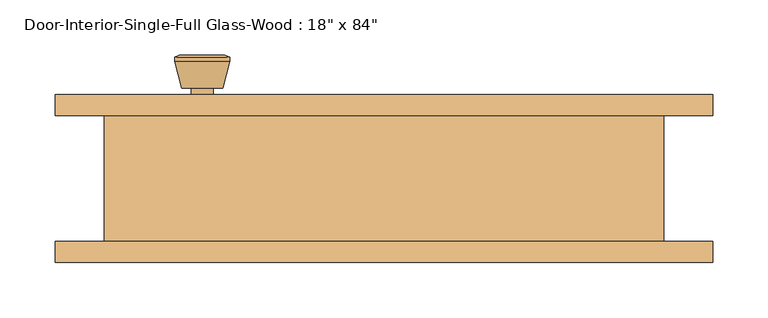
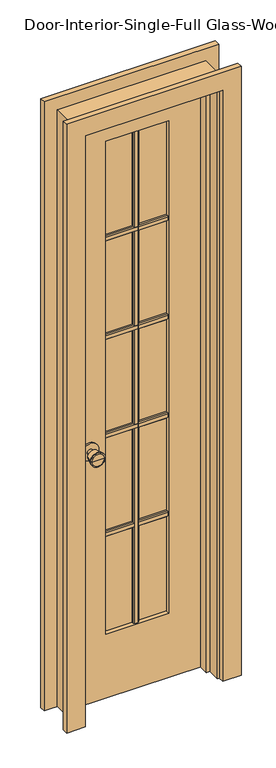
"""IFC4 building model written with IfcOpenShell, lengths in millimetres: door geometry."""

from ifc_helpers import new_model, si_unit, point, frame, frame_2d, origin, place, context, project, spatial, polyline, circle_curve, trimmed, segment, composite_curve, outline, extrude, faceted_brep, source, transform, mapped, element, save
from ifc_brep_helpers import plane_surface, cylinder_surface, revolved_surface, advanced_brep


def door_ccf0cbd1(model_context):
    return source(origin(), model_context, "Body", "SolidModel", [
        extrude(outline(polyline([(40.005, 1667.51), (46.355, 1667.51), (49.53, 1664.335), (49.53, 1651.635), (46.355, 1648.46), (40.005, 1648.46), (40.005, 1667.51)])), frame((-107.95, 0.0, 0.0), z_axis=(1.0, 0.0, 0.0), x_axis=(0.0, 1.0, 0.0)), (0.0, 0.0, 1.0), 215.9),
        extrude(outline(polyline([(40.005, 1310.9575), (46.355, 1310.9575), (49.53, 1307.7825), (49.53, 1295.0825), (46.355, 1291.9075), (40.005, 1291.9075), (40.005, 1310.9575)])), frame((-107.95, 0.0, 0.0), z_axis=(1.0, 0.0, 0.0), x_axis=(0.0, 1.0, 0.0)), (0.0, 0.0, 1.0), 215.9),
        extrude(outline(polyline([(40.005, 954.405), (46.355, 954.405), (49.53, 951.23), (49.53, 938.53), (46.355, 935.355), (40.005, 935.355), (40.005, 954.405)])), frame((-107.95, 0.0, 0.0), z_axis=(1.0, 0.0, 0.0), x_axis=(0.0, 1.0, 0.0)), (0.0, 0.0, 1.0), 215.9),
        extrude(outline(polyline([(-9.525, 40.005), (-9.525, 46.355), (-6.35, 49.53), (6.35, 49.53), (9.525, 46.355), (9.525, 40.005), (-9.525, 40.005)])), frame((0.0, 0.0, 231.775), z_axis=(0.0, 0.0, 1.0), x_axis=(1.0, 0.0, 0.0)), (0.0, 0.0, 1.0), 1782.7625),
        extrude(outline(polyline([(40.005, 597.8525), (46.355, 597.8525), (49.53, 594.6775), (49.53, 581.9775), (46.355, 578.8025), (40.005, 578.8025), (40.005, 597.8525)])), frame((-107.95, 0.0, 0.0), z_axis=(1.0, 0.0, 0.0), x_axis=(0.0, 1.0, 0.0)), (0.0, 0.0, 1.0), 215.9),
        extrude(outline(polyline([(33.02, 1667.51), (33.02, 1648.46), (26.67, 1648.46), (23.495, 1651.635), (23.495, 1664.335), (26.67, 1667.51), (33.02, 1667.51)])), frame((-107.95, 0.0, 0.0), z_axis=(1.0, 0.0, 0.0), x_axis=(0.0, 1.0, 0.0)), (0.0, 0.0, 1.0), 215.9),
        extrude(outline(polyline([(33.02, 1310.9575), (33.02, 1291.9075), (26.67, 1291.9075), (23.495, 1295.0825), (23.495, 1307.7825), (26.67, 1310.9575), (33.02, 1310.9575)])), frame((-107.95, 0.0, 0.0), z_axis=(1.0, 0.0, 0.0), x_axis=(0.0, 1.0, 0.0)), (0.0, 0.0, 1.0), 215.9),
        extrude(outline(polyline([(33.02, 954.405), (33.02, 935.355), (26.67, 935.355), (23.495, 938.53), (23.495, 951.23), (26.67, 954.405), (33.02, 954.405)])), frame((-107.95, 0.0, 0.0), z_axis=(1.0, 0.0, 0.0), x_axis=(0.0, 1.0, 0.0)), (0.0, 0.0, 1.0), 215.9),
        extrude(outline(polyline([(-9.525, 33.02), (9.525, 33.02), (9.525, 26.67), (6.35, 23.495), (-6.35, 23.495), (-9.525, 26.67), (-9.525, 33.02)])), frame((0.0, 0.0, 231.775), z_axis=(0.0, 0.0, 1.0), x_axis=(1.0, 0.0, 0.0)), (0.0, 0.0, 1.0), 1782.7625),
        extrude(outline(polyline([(33.02, 597.8525), (33.02, 578.8025), (26.67, 578.8025), (23.495, 581.9775), (23.495, 594.6775), (26.67, 597.8525), (33.02, 597.8525)])), frame((-107.95, 0.0, 0.0), z_axis=(1.0, 0.0, 0.0), x_axis=(0.0, 1.0, 0.0)), (0.0, 0.0, 1.0), 215.9),
        advanced_brep(
        [(-165.1, 13.05, 914.4), (-155.1, 13.05, 914.4), (-175.1, 13.05, 914.4), (-144.6241324, -35.95, 914.4), (-165.1, -35.95, 914.4), (-185.5758676, -35.95, 914.4), (-140.1, -34.1221319, 914.4), (-190.1, -34.1221319, 914.4), (-140.1, -30.6584537, 914.4), (-190.1, -30.6584537, 914.4), (-146.463764, -5.95, 914.4), (-183.736236, -5.95, 914.4), (-155.1, -5.95, 914.4), (-175.1, -5.95, 914.4)],
        [
            (0, 1),
            (1, 2, circle_curve(frame((-165.1, 13.05, 914.4), z_axis=(0.0, 1.0, 0.0), x_axis=(-1.0, 0.0, 0.0)), 10.0)),
            (2, 0),
            (2, 1, circle_curve(frame((-165.1, 13.05, 914.4), z_axis=(0.0, 1.0, 0.0), x_axis=(-1.0, 0.0, 0.0)), 10.0)),
            (3, 4),
            (4, 5),
            (5, 3, circle_curve(frame((-165.1, -35.95, 914.4), z_axis=(0.0, -1.0, 0.0), x_axis=(-1.0, 0.0, 0.0)), 20.4758676)),
            (3, 5, circle_curve(frame((-165.1, -35.95, 914.4), z_axis=(0.0, -1.0, 0.0), x_axis=(-1.0, 0.0, 0.0)), 20.4758676)),
            (6, 3),
            (5, 7),
            (7, 6, circle_curve(frame((-165.1, -34.1221319, 914.4), z_axis=(0.0, -1.0, 0.0), x_axis=(-1.0, 0.0, 0.0)), 25.0)),
            (6, 7, circle_curve(frame((-165.1, -34.1221319, 914.4), z_axis=(0.0, -1.0, 0.0), x_axis=(-1.0, 0.0, 0.0)), 25.0)),
            (8, 6),
            (7, 9),
            (9, 8, circle_curve(frame((-165.1, -30.6584537, 914.4), z_axis=(0.0, -1.0, 0.0), x_axis=(-1.0, 0.0, 0.0)), 25.0)),
            (8, 9, circle_curve(frame((-165.1, -30.6584537, 914.4), z_axis=(0.0, -1.0, 0.0), x_axis=(-1.0, 0.0, 0.0)), 25.0)),
            (10, 8),
            (9, 11),
            (11, 10, circle_curve(frame((-165.1, -5.95, 914.4), z_axis=(0.0, -1.0, 0.0), x_axis=(-1.0, 0.0, 0.0)), 18.636236)),
            (10, 11, circle_curve(frame((-165.1, -5.95, 914.4), z_axis=(0.0, -1.0, 0.0), x_axis=(-1.0, 0.0, 0.0)), 18.636236)),
            (12, 10),
            (11, 13),
            (13, 12, circle_curve(frame((-165.1, -5.95, 914.4), z_axis=(0.0, -1.0, 0.0), x_axis=(-1.0, 0.0, 0.0)), 10.0)),
            (12, 13, circle_curve(frame((-165.1, -5.95, 914.4), z_axis=(0.0, -1.0, 0.0), x_axis=(-1.0, 0.0, 0.0)), 10.0)),
            (1, 12),
            (13, 2),
        ],
        [
            plane_surface(frame((-165.1, 13.05, 914.4), z_axis=(0.0, 1.0, 0.0), x_axis=(-1.0, 0.0, 0.0))),
            plane_surface(frame((-165.1, -35.95, 914.4), z_axis=(0.0, -1.0, 0.0), x_axis=(-1.0, 0.0, 0.0))),
            revolved_surface(polyline([(-185.5758676, -35.95, 914.4), (-190.1, -34.1221319, 914.4)]), (-165.1, 13.05, 914.4), (0.0, 1.0, 0.0)),
            cylinder_surface(frame((-165.1, 13.05, 914.4), z_axis=(0.0, 1.0, 0.0), x_axis=(-1.0, 0.0, 0.0)), 25.0),
            revolved_surface(polyline([(-190.1, -30.6584537, 914.4), (-183.736236, -5.95, 914.4)]), (-165.1, 13.05, 914.4), (0.0, 1.0, 0.0)),
            plane_surface(frame((-165.1, -5.95, 914.4), z_axis=(0.0, 1.0, 0.0), x_axis=(-1.0, 0.0, 0.0))),
            cylinder_surface(frame((-165.1, 13.05, 914.4), z_axis=(0.0, 1.0, 0.0), x_axis=(-1.0, 0.0, 0.0)), 10.0),
        ],
        [
            (0, [[1, 2, 3]]),
            (0, [[-3, 4, -1]]),
            (1, [[5, 6, 7]]),
            (1, [[-6, -5, 8]]),
            (2, [[9, -7, 10, 11]]),
            (2, [[-10, -8, -9, 12]]),
            (3, [[13, -11, 14, 15]]),
            (3, [[-14, -12, -13, 16]]),
            (4, [[17, -15, 18, 19]]),
            (4, [[-18, -16, -17, 20]]),
            (5, [[21, -19, 22, 23]]),
            (5, [[-22, -20, -21, 24]]),
            (6, [[25, -23, 26, -2]]),
            (6, [[-26, -24, -25, -4]]),
        ],
    ),
        extrude(outline(composite_curve([segment(trimmed(circle_curve(frame_2d((914.4, -165.1)), 30.0), [point((914.4, -195.1))], [point((914.4, -135.1))], False, "CARTESIAN"), True, "CONTINUOUS"), segment(trimmed(circle_curve(frame_2d((914.4, -165.1)), 30.0), [point((914.4, -135.1))], [point((914.4, -195.1))], False, "CARTESIAN"), True, "CONTINUOUS")], self_intersect=False)), frame((0.0, 13.05, 0.0), z_axis=(0.0, 1.0, 0.0), x_axis=(0.0, 0.0, 1.0)), (0.0, 0.0, 1.0), 6.0),
        advanced_brep(
        [(-165.1, 59.975, 914.4), (-175.1, 59.975, 914.4), (-155.1, 59.975, 914.4), (-144.6241324, 108.975, 914.4), (-185.5758676, 108.975, 914.4), (-165.1, 108.975, 914.4), (-140.1, 107.1471319, 914.4), (-190.1, 107.1471319, 914.4), (-140.1, 103.6834537, 914.4), (-190.1, 103.6834537, 914.4), (-146.463764, 78.975, 914.4), (-183.736236, 78.975, 914.4), (-155.1, 78.975, 914.4), (-175.1, 78.975, 914.4)],
        [
            (0, 1),
            (1, 2, circle_curve(frame((-165.1, 59.975, 914.4), z_axis=(0.0, -1.0, 0.0), x_axis=(-1.0, 0.0, 0.0)), 10.0)),
            (2, 0),
            (2, 1, circle_curve(frame((-165.1, 59.975, 914.4), z_axis=(0.0, -1.0, 0.0), x_axis=(-1.0, 0.0, 0.0)), 10.0)),
            (3, 4, circle_curve(frame((-165.1, 108.975, 914.4), z_axis=(0.0, 1.0, 0.0), x_axis=(-1.0, 0.0, 0.0)), 20.4758676)),
            (4, 5),
            (5, 3),
            (4, 3, circle_curve(frame((-165.1, 108.975, 914.4), z_axis=(0.0, 1.0, 0.0), x_axis=(-1.0, 0.0, 0.0)), 20.4758676)),
            (6, 7, circle_curve(frame((-165.1, 107.1471319, 914.4), z_axis=(0.0, 1.0, 0.0), x_axis=(-1.0, 0.0, 0.0)), 25.0)),
            (7, 4),
            (3, 6),
            (7, 6, circle_curve(frame((-165.1, 107.1471319, 914.4), z_axis=(0.0, 1.0, 0.0), x_axis=(-1.0, 0.0, 0.0)), 25.0)),
            (8, 9, circle_curve(frame((-165.1, 103.6834537, 914.4), z_axis=(0.0, 1.0, 0.0), x_axis=(-1.0, 0.0, 0.0)), 25.0)),
            (9, 7),
            (6, 8),
            (9, 8, circle_curve(frame((-165.1, 103.6834537, 914.4), z_axis=(0.0, 1.0, 0.0), x_axis=(-1.0, 0.0, 0.0)), 25.0)),
            (10, 11, circle_curve(frame((-165.1, 78.975, 914.4), z_axis=(0.0, 1.0, 0.0), x_axis=(-1.0, 0.0, 0.0)), 18.636236)),
            (11, 9),
            (8, 10),
            (11, 10, circle_curve(frame((-165.1, 78.975, 914.4), z_axis=(0.0, 1.0, 0.0), x_axis=(-1.0, 0.0, 0.0)), 18.636236)),
            (12, 13, circle_curve(frame((-165.1, 78.975, 914.4), z_axis=(0.0, 1.0, 0.0), x_axis=(-1.0, 0.0, 0.0)), 10.0)),
            (13, 11),
            (10, 12),
            (13, 12, circle_curve(frame((-165.1, 78.975, 914.4), z_axis=(0.0, 1.0, 0.0), x_axis=(-1.0, 0.0, 0.0)), 10.0)),
            (1, 13),
            (12, 2),
        ],
        [
            plane_surface(frame((-165.1, 59.975, 914.4), z_axis=(0.0, -1.0, 0.0), x_axis=(-1.0, 0.0, 0.0))),
            plane_surface(frame((-165.1, 108.975, 914.4), z_axis=(0.0, 1.0, 0.0), x_axis=(-1.0, 0.0, 0.0))),
            revolved_surface(polyline([(-185.5758676, 108.975, 914.4), (-190.1, 107.1471319, 914.4)]), (-165.1, 59.975, 914.4), (0.0, -1.0, 0.0)),
            cylinder_surface(frame((-165.1, 59.975, 914.4), z_axis=(0.0, -1.0, 0.0), x_axis=(-1.0, 0.0, 0.0)), 25.0),
            revolved_surface(polyline([(-190.1, 103.6834537, 914.4), (-183.736236, 78.975, 914.4)]), (-165.1, 59.975, 914.4), (0.0, -1.0, 0.0)),
            plane_surface(frame((-165.1, 78.975, 914.4), z_axis=(0.0, -1.0, 0.0), x_axis=(-1.0, 0.0, 0.0))),
            cylinder_surface(frame((-165.1, 59.975, 914.4), z_axis=(0.0, -1.0, 0.0), x_axis=(-1.0, 0.0, 0.0)), 10.0),
        ],
        [
            (0, [[1, 2, 3]]),
            (0, [[-3, 4, -1]]),
            (1, [[5, 6, 7]]),
            (1, [[8, -7, -6]]),
            (2, [[9, 10, -5, 11]]),
            (2, [[12, -11, -8, -10]]),
            (3, [[13, 14, -9, 15]]),
            (3, [[16, -15, -12, -14]]),
            (4, [[17, 18, -13, 19]]),
            (4, [[20, -19, -16, -18]]),
            (5, [[21, 22, -17, 23]]),
            (5, [[24, -23, -20, -22]]),
            (6, [[-2, 25, -21, 26]]),
            (6, [[-4, -26, -24, -25]]),
        ],
    ),
        extrude(outline(composite_curve([segment(trimmed(circle_curve(frame_2d((914.4, -165.1)), 30.0), [point((914.4, -195.1))], [point((914.4, -135.1))], False, "CARTESIAN"), True, "CONTINUOUS"), segment(trimmed(circle_curve(frame_2d((914.4, -165.1)), 30.0), [point((914.4, -135.1))], [point((914.4, -195.1))], False, "CARTESIAN"), True, "CONTINUOUS")], self_intersect=False)), frame((0.0, 53.975, 0.0), z_axis=(0.0, 1.0, 0.0), x_axis=(0.0, 0.0, 1.0)), (0.0, 0.0, 1.0), 6.0),
        faceted_brep([(254.0, 53.975, 0.0), (254.0, -60.325, 0.0), (228.6, -60.325, 0.0), (228.6, -15.875, 0.0), (215.9, -15.875, 0.0), (215.9, 19.05, 0.0), (228.6, 19.05, 0.0), (228.6, 53.975, 0.0), (254.0, 53.975, 2159.0), (254.0, -60.325, 2159.0), (-254.0, -60.325, 2159.0), (-254.0, -60.325, 0.0), (-228.6, -60.325, 0.0), (-228.6, -60.325, 2133.6), (228.6, -60.325, 2133.6), (228.6, -15.875, 2133.6), (-228.6, -15.875, 2133.6), (-228.6, -15.875, 0.0), (-215.9, -15.875, 0.0), (-215.9, -15.875, 2120.9), (215.9, -15.875, 2120.9), (215.9, 19.05, 2120.9), (-215.9, 19.05, 2120.9), (-215.9, 19.05, 0.0), (-228.6, 19.05, 0.0), (-228.6, 19.05, 2133.6), (228.6, 19.05, 2133.6), (228.6, 53.975, 2133.6), (-228.6, 53.975, 2133.6), (-228.6, 53.975, 0.0), (-254.0, 53.975, 0.0), (-254.0, 53.975, 2159.0)], [[[0, 1, 2, 3, 4, 5, 6, 7]], [[1, 0, 8, 9]], [[2, 1, 9, 10, 11, 12, 13, 14]], [[3, 2, 14, 15]], [[4, 3, 15, 16, 17, 18, 19, 20]], [[5, 4, 20, 21]], [[6, 5, 21, 22, 23, 24, 25, 26]], [[7, 6, 26, 27]], [[0, 7, 27, 28, 29, 30, 31, 8]], [[9, 8, 31, 10]], [[15, 14, 13, 16]], [[21, 20, 19, 22]], [[27, 26, 25, 28]], [[30, 29, 24, 23, 18, 17, 12, 11]], [[10, 31, 30, 11]], [[16, 13, 12, 17]], [[22, 19, 18, 23]], [[28, 25, 24, 29]]]),
        extrude(outline(polyline([(2133.6, -228.6), (0.0, -228.6), (0.0, 228.6), (2133.6, 228.6), (2133.6, -228.6)]), holes=[polyline([(2014.5375, -107.95), (2014.5375, 107.95), (231.775, 107.95), (231.775, -107.95), (2014.5375, -107.95)])]), frame((0.0, 19.05, 0.0), z_axis=(0.0, 1.0, 0.0), x_axis=(0.0, 0.0, 1.0)), (0.0, 0.0, 1.0), 34.925),
        extrude(outline(polyline([(107.95, 33.02), (-107.95, 33.02), (-107.95, 40.005), (107.95, 40.005), (107.95, 33.02)])), frame((0.0, 0.0, 231.775), z_axis=(0.0, 0.0, 1.0), x_axis=(1.0, 0.0, 0.0)), (0.0, 0.0, 1.0), 1782.7625),
        extrude(outline(polyline([(0.0, 234.95), (0.0, 298.45), (2203.45, 298.45), (2203.45, -298.45), (0.0, -298.45), (0.0, -234.95), (2139.95, -234.95), (2139.95, 234.95), (0.0, 234.95)])), frame((0.0, 53.975, 0.0), z_axis=(0.0, 1.0, 0.0), x_axis=(0.0, 0.0, 1.0)), (0.0, 0.0, 1.0), 19.05),
        extrude(outline(polyline([(0.0, 234.95), (0.0, 298.45), (2203.45, 298.45), (2203.45, -298.45), (0.0, -298.45), (0.0, -234.95), (2139.95, -234.95), (2139.95, 234.95), (0.0, 234.95)])), frame((0.0, -79.375, 0.0), z_axis=(0.0, 1.0, 0.0), x_axis=(0.0, 0.0, 1.0)), (0.0, 0.0, 1.0), 19.05),
    ])


if __name__ == "__main__":
    model = new_model("IFC4")
    model_context = context("Model", 3, world=origin())
    ifc_project = project(units=[si_unit("LENGTHUNIT", "METRE", prefix="MILLI")], contexts=[model_context])
    site = spatial("IfcSite", under=ifc_project)
    building = spatial("IfcBuilding", under=site)
    placement = place(None, origin())
    door_shape = door_ccf0cbd1(model_context)
    element("IfcDoor", 1, ObjectType="Door-Interior-Single-Full Glass-Wood : 18\" x 84\"", at=placement, inside=building, context=model_context, shape_type="MappedRepresentation", body=[
        mapped(door_shape, transform((0.0, 0.0, 0.0), x_axis=(1.0, 0.0, 0.0), y_axis=(0.0, 1.0, 0.0), z_axis=(0.0, 0.0, 1.0))),
    ])
    save(model, "model.ifc")

# Revit data of these elements
# Type "Door-Interior-Single-Full Glass-Wood : 18\" x 84\""
#   Type Mark = "13"
#   Assembly Code = "C1020300"
#   Analytic Construction = "Wood frame with single clear glass"
#   Top Rail = 0' - 4 11/16"
#   Thickness = 0' - 1 3/8"
#   Thermal Resistance (R) = 1.0102 (h·ft²·°F)/BTU
#   Swing Angle [instance default] = 90.00°
#   Stiles = 0' - 4 3/4"
#   Rough Width = 1' - 8"
#   Rough Height = 7' - 1"
#   Height = 7' - 0"
#   Width = 1' - 6"
#   Heat Transfer Coefficient (U) = 0.9900 BTU/(h·ft²·°F)
#   Bottom Rail = 0' - 9 1/8"
#   Show Grill [instance default] = yes
#   Trim Material = Cherry
#   Panel Material = Cherry
#   Frame Material = Cherry
#   Door Handle Material = Aluminum
#   Visual Light Transmittance = 0
#   Solar Heat Gain Coefficient = 0
#   Wall Closure = (empty or 0)
#   Function = (empty or 0)
# Element 1 (IfcDoor, "Door-Interior-Single-Full Glass-Wood : 18\" x 84\"")
#   Materials on its faces: "Cherry", "Aluminum", "Glass"
# Materials
#   "Cherry": class "Wood", colour RGB 226 177 128, transparency 0, Description = "Prunus Serotina", Cost = 0
#   "Aluminum": class "Metal", colour RGB 247 247 247, transparency 0, Description = "Aluminum 6061", Cost = 0
#   "Glass": class "Glass", colour RGB 0 128 192, transparency 0.75, Description = "Soda Lime Glass", Cost = 0
